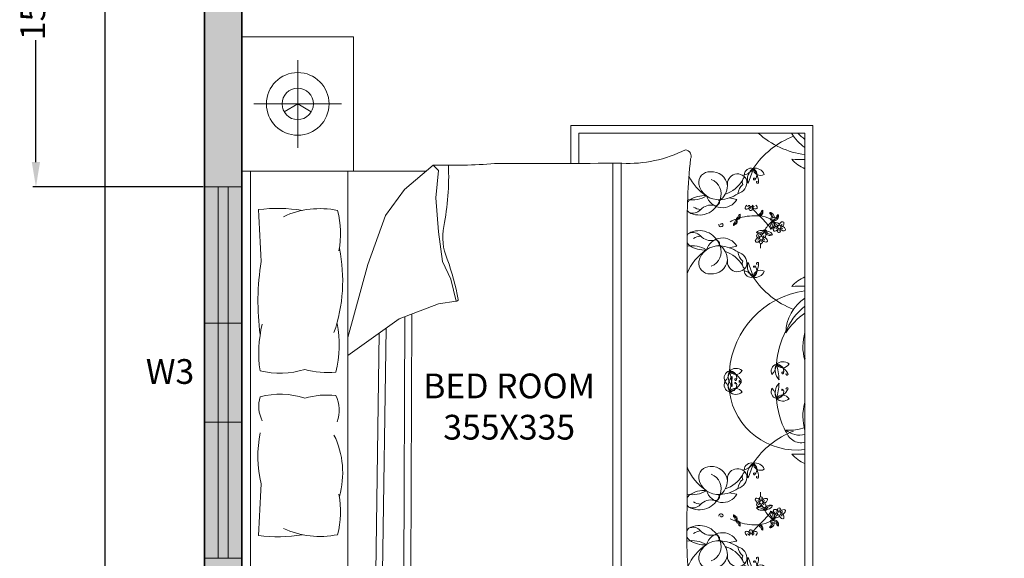
# Model space of a CAD drawing. Units: centimetres. Extents: x 2401 to 3632, y 2122 to 3526.
# Tile 2 of 10: x 2426 to 2824, y 2374 to 2591. Entities that reach past the tile are written whole.
import ezdxf

# ---------------------------------------------------------------- set-up
doc = ezdxf.new("R2010")
doc.units = ezdxf.units.CM
for name, color, linetype, lineweight in [('A-ANNO-DIMS', 9, 'Continuous', 18), ('A-ANNO-TEXT', 9, 'Continuous', 18), ('A-AREA-IDEN', 9, 'Continuous', 25), ('A-FURN', 9, 'Continuous', 18), ('A-GLAZ', 4, 'Continuous', 18), ('A-WALL', 7, 'Continuous', 35)]:
    doc.layers.add(name, color=color, linetype=linetype, lineweight=lineweight)
doc.layers.add('A-GLAZ-PATT', color=251, linetype='Continuous', lineweight=13, true_color=0x636466)
doc.layers.add('A-WALL-PATT', color=18, linetype='Continuous', lineweight=13, true_color=0x000000)
doc.styles.get("Standard").update_dxf_attribs({"font": 'arial.ttf'})
doc.dimstyles.new('ISO-25', dxfattribs={"dimtxt": 10, "dimasz": 10, "dimexe": 1.25, "dimexo": 0.625, "dimtad": 0, "dimtxsty": 'Standard', "dimcen": 2.5, "dimadec": 0, "dimazin": 0, "dimtfac": 1, "dimtmove": 0, "dimatfit": 3, "dimfxl": 1, "dimarcsym": 0})

# ---------------------------------------------------------------- blocks, each defined once
blk = doc.blocks.new('bed')
for p, q in [((3025.77, 3949.95), (3025.77, 3649.95)), ((3000.77, 3900.35), (3000.77, 3939.55)), ((2981.17, 3919.95), (3020.37, 3919.95)), ((2770.64, 3910.36), (2878.71, 3910.36)), ((2770.64, 3691.65), (2770.64, 3910.36)), ((2774.11, 3906.88), (2774.11, 3695.12)), ((2875.23, 3906.88), (2774.11, 3906.88)), ((2875.23, 3893.39), (2875.23, 3906.88)), ((2878.71, 3910.36), (2878.71, 3893.39)), ((2856.25, 3708.31), (2856.25, 3893.41)), ((2860, 3708.59), (2860, 3893.41)), ((2937.86, 3890.21), (2940.29, 3892.64)), ((2939.08, 3878.06), (2937.86, 3890.21)), ((2940.29, 3892.64), (2953.05, 3881.7)), ((3025.77, 3889.95), (2943.43, 3889.95)), ((2978.36, 3889.95), (2978.36, 3709.95)), ((3021.92, 3709.95), (3021.92, 3889.95)), ((2953.05, 3881.7), (2961.55, 3870.16)), ((2804.53, 3877.32), (2807.92, 3877.98)), ((2937.86, 3862.87), (2939.08, 3878.06)), ((2961.55, 3870.16), (2969.44, 3848.28)), ((2936.04, 3849.5), (2937.86, 3862.87)), ((2826.78, 3739.05), (2826.78, 3860.86)), ((2804.53, 3856.35), (2807.92, 3855.69)), ((2932.4, 3841.6), (2936.04, 3849.5)), ((2969.44, 3848.28), (2978.36, 3815.57)), ((2929.97, 3831.88), (2932.4, 3841.6)), ((2937.86, 3830.66), (2929.97, 3831.88)), ((2955.47, 3823.98), (2937.86, 3830.66)), ((2950.29, 3711.02), (2949.82, 3826.13)), ((2953.37, 3711.03), (2952.92, 3824.95)), ((2978.36, 3807.54), (2955.47, 3823.98)), ((2962.82, 3710.88), (2961.28, 3819.81)), ((2965.89, 3710.76), (2964.4, 3817.57)), ((2804.53, 3745.65), (2807.92, 3746.31)), ((2804.53, 3724.68), (2807.92, 3724.02)), ((2875.23, 3695.12), (2875.23, 3708.35)), ((2878.71, 3708.28), (2878.71, 3691.65)), ((3000.77, 3699.55), (3000.77, 3660.35)), ((2878.71, 3691.65), (2770.64, 3691.65)), ((2774.11, 3695.12), (2875.23, 3695.12)), ((2981.17, 3679.95), (3020.37, 3679.95))]:
    blk.add_line(p, q)
for points in [[(2975.77, 3889.95), (2975.77, 3949.95), (3025.77, 3949.95)], [(3000.77, 3919.95), (2994.7, 3916.45)], [(3000.77, 3919.95), (3006.83, 3916.45)], [(3025.77, 3709.95), (2975.77, 3709.95), (2975.77, 3649.95), (3025.77, 3649.95)], [(3000.77, 3679.95), (2994.7, 3683.45)], [(3000.77, 3679.95), (3006.83, 3683.45)]]:
    blk.add_lwpolyline(points)
for points in [[(2912.82, 3893.27, 0.001242), (2855.9, 3893.41, -0.127202), (2827.53, 3899.43)], [(3018.29, 3872.72, 0.074897), (2998.69, 3872.36, -0.472817)], [(2997.6, 3801.36, 0.14099), (3017.59, 3800.76, 0.235245)], [(2997.6, 3788.55, -0.14099), (3017.59, 3789.15, -0.235245)], [(3018.29, 3727.19, -0.074897), (2998.69, 3727.55, 0.472817)], [(2862.36, 3708.67, 0.056112), (2845.85, 3706.5, 0.095341), (2829.95, 3702.28)]]:
    blk.add_lwpolyline(points, format="xyb")
for centre, radius in [((3000.77, 3919.95), 14), ((3000.77, 3919.95), 7), ((2785.6, 3864.98), 0.764), ((2793.66, 3859.99), 0.764), ((2793.66, 3742.02), 0.764), ((2785.6, 3737.02), 0.764), ((3000.77, 3679.95), 14), ((3000.77, 3679.95), 7)]:
    blk.add_circle(centre, radius)
for centre, radius, start, end in [((2760.03, 3923.26), 23.79, 306.3036, 316.4814), ((2763.59, 3916.39), 19.09, 303.4617, 330.1116), ((2768.83, 3936.05), 39.18, 277.745, 311.8856), ((2764.96, 3869.02), 39.18, 34.3865, 68.5908), ((2827.73, 3896.66), 2.77, 93.98, 207.3412), ((2768, 3905.7), 15.93, 292.5547, 318.9546), ((2776.56, 3949.33), 54.2, 267.4081, 273.6519), ((2514.5, 3864.44), 312.3, 359.3433, 5.6887), ((2796.37, 3886.9), 4.34, 77.7115, 159.0387), ((2794.02, 3891.25), 3.27, 238.4633, 358.2869), ((2804.75, 3884.63), 9.91, 138.8402, 177.9352), ((2798.78, 3888.31), 3.2, 117.6827, 223.7762), ((2798.06, 3887.99), 3.25, 2.9516, 103.728), ((2824.04, 3897.09), 27.41, 192.5173, 207.1824), ((2793.67, 3886.12), 6.19, 345.4653, 54.2343), ((2803, 3894.63), 6.69, 211.3827, 255.2969), ((2815.84, 3882.53), 7.17, 84.9449, 172.8857), ((2816.56, 3884.61), 5.07, 354.4856, 91.0538), ((2932.84, 4167.71), 275.17, 265.8294, 271.553), ((3046.53, 3887.51), 113.22, 177.4519, 191.3392), ((2795.33, 3884.97), 0.487, 177.9352, 11.4834), ((2795.58, 3885.02), 0.236, 11.4834, 127.9409), ((2796.77, 3886.39), 0.424, 223.7762, 159.7183), ((2805.64, 3885.26), 5.62, 175.969, 254.3045), ((2804.28, 3884.18), 4.5, 350.264, 160.8688), ((2799.41, 3885.11), 2.76, 333.9755, 53.2681), ((2814.2, 3893.11), 14.16, 211.2614, 251.7045), ((2818.55, 3879.71), 6.96, 111.5819, 201.4221), ((2805.66, 3897.83), 22.71, 303.6671, 333.2997), ((2798.17, 3879.2), 5.99, 6.1662, 51.5825), ((2817.43, 3883.78), 8.71, 182.3591, 234.0401), ((2812.81, 3886.16), 9.02, 265.2933, 346.921), ((2813.05, 3893.24), 16.1, 236.2883, 266.5076), ((2810.99, 3881.04), 7.46, 209.9085, 343.1337), ((2814.13, 3876.31), 1.86, 167.3041, 285.1471), ((2819.17, 3867.4), 11.57, 122.7011, 126.3445), ((2821.34, 3879.88), 9.56, 199.2822, 299.1751), ((2824.57, 3889.51), 12.43, 238.8218, 279.1554), ((2819.17, 3867.4), 11.57, 55.785, 94.7304), ((2823.47, 3874.11), 3.61, 30.0293, 52.325), ((2789.51, 3870.54), 0.853, 56.8636, 146.9021), ((2801.41, 3872.25), 8.46, 178.3264, 187.1302), ((2792.27, 3871.07), 1.58, 11.3256, 64.4621), ((2797.62, 3873.34), 4.74, 190.2588, 210.656), ((2797.6, 3874.36), 4.82, 218.2101, 226.3071), ((2775.06, 3890.75), 28.48, 313.1541, 322.0459), ((2796.01, 3873.64), 0.586, 142.4737, 265.053), ((2796.78, 3873.76), 1.26, 127.7621, 169.0403), ((2796.11, 3874.82), 1.78, 265.053, 338.3618), ((2798.46, 3872.39), 2.32, 113.4276, 137.6104), ((2798.2, 3874.8), 0.764, 183.2768, 356.7232), ((2798.76, 3873.41), 1.25, 139.7889, 227.6792), ((2798.36, 3872.98), 0.658, 227.6792, 350.3487), ((2795.81, 3873.43), 2.5, 353.0852, 15.7171), ((2797.45, 3873.13), 1.58, 350.3487, 43.6538), ((2800.38, 3874.76), 1.84, 198.7263, 262.5032), ((2798.92, 3873.91), 0.73, 1.1081, 91.8675), ((2800.29, 3873.51), 0.59, 255.2356, 54.9248), ((2799.38, 3873.74), 1.27, 11.5637, 52.6358), ((2816.22, 3868.58), 6.15, 41.5653, 105.1471), ((2819.61, 3881.32), 8.62, 277.436, 299.9149), ((2824.18, 3875.64), 4.49, 221.5653, 293.8354), ((2823.47, 3874.11), 3.61, 314.4517, 333.558), ((3021.8, 3862.02), 40.2, 165.1039, 191.0369), ((2990.83, 3834.5), 38.67, 65.1316, 101.7583), ((5873.3, 3707.37), 2859.79, 176.68521, 177.14978), ((2785.02, 3866.54), 1.51, 157.4086, 261.4386), ((2784.17, 3866.59), 0.757, 58.0499, 135.6268), ((2783.3, 3865.19), 2.41, 14.7558, 58.0499), ((2786.72, 3869.91), 0.853, 124.3538, 214.3923), ((2787.97, 3869.78), 1.99, 190.3057, 287.1958), ((2788.54, 3870.49), 2.31, 176.9701, 248.2913), ((2805.02, 3882.67), 22.32, 212.6784, 216.3746), ((2787.76, 3869.95), 0.883, 216.3746, 291.7548), ((2795.58, 3857.56), 12.46, 124.0033, 132.4917), ((2782.77, 3855.98), 13.31, 63.7819, 68.2913), ((2789.87, 3866.22), 2.12, 128.3208, 208.8162), ((2789.87, 3869.34), 1.99, 122.8155, 187.3992), ((2788.34, 3868.51), 0.666, 289.3605, 111.7548), ((2788.84, 3868.51), 0.666, 221.8703, 44.2646), ((2791.86, 3866.57), 3.48, 157.2305, 229.0635), ((2790.75, 3869.08), 2.31, 109.4799, 177.6828), ((2790.69, 3867.72), 2.05, 174.4544, 220.6188), ((2779.03, 3856.28), 14.94, 30.544, 49.818), ((2789.95, 3869.59), 0.883, 148.8844, 224.2646), ((2808.3, 3858.51), 22.32, 145.1882, 148.8844), ((2795.58, 3857.56), 12.46, 94.756, 119.2041), ((2822.1, 3839.62), 40.99, 132.2412, 142.1744), ((2794.44, 3871.41), 1.44, 188.3432, 274.2869), ((2795.7, 3872.2), 2.51, 210.656, 242.6341), ((2794.04, 3870.31), 0.611, 325.7657, 67.4417), ((2796.2, 3845.18), 24.85, 73.5842, 93.8277), ((2811.5, 3870.46), 8.46, 178.3264, 187.1302), ((2802.37, 3869.29), 1.58, 11.3256, 64.4621), ((2807.71, 3871.55), 4.74, 190.2588, 210.656), ((2804.53, 3869.62), 1.44, 188.3432, 274.2869), ((2805.8, 3870.42), 2.51, 210.656, 242.6341), ((2807.7, 3872.58), 4.82, 218.2101, 226.3071), ((2804.13, 3868.53), 0.611, 325.7657, 67.4417), ((2805.85, 3867.41), 1.44, 147.5332, 233.4768), ((2804.7, 3867.58), 0.611, 354.3784, 96.0543), ((2807.15, 3868.15), 2.51, 179.1859, 211.164), ((2796.2, 3845.18), 24.85, 63.0032, 69.8941), ((2809.96, 3868.8), 4.82, 195.5129, 203.6099), ((2783.42, 3863.83), 0.586, 142.4737, 265.053), ((2784.19, 3863.94), 1.26, 61.2196, 169.0403), ((2783.52, 3865.01), 1.78, 265.053, 338.3618), ((2785.87, 3862.58), 2.32, 113.4276, 137.6104), ((2784.96, 3866.11), 0.506, 172.906, 277.132), ((2786.17, 3863.6), 1.25, 139.7889, 227.6792), ((2785.77, 3863.16), 0.658, 227.6792, 350.3487), ((2786.67, 3865.83), 1.04, 36.1046, 181.4281), ((2783.22, 3863.62), 2.5, 353.0852, 15.7171), ((2784.86, 3863.32), 1.58, 350.3487, 43.6538), ((2787.79, 3864.95), 1.84, 198.7263, 262.5032), ((2786.06, 3866.65), 1.05, 270.0645, 331.1507), ((2786.96, 3866.4), 1.2, 221.8413, 265.7877), ((2786.33, 3864.09), 0.73, 1.1081, 91.8675), ((2786.95, 3865.94), 0.749, 263.7526, 41.7054), ((2786.79, 3863.93), 1.27, 11.5637, 86.365), ((2787.7, 3863.7), 0.59, 255.2356, 54.9248), ((2790.26, 3866.38), 2.53, 207.7043, 254.3516), ((2788.61, 3864.93), 3.48, 270.278, 342.111), ((2790.93, 3860.58), 2.46, 98.7227, 159.3375), ((2787.26, 3864.79), 2.46, 340.0041, 40.6188), ((2790.25, 3865.04), 2.05, 278.7227, 324.8872), ((2789.89, 3863.37), 2.12, 290.5253, 358.5375), ((2794.02, 3863.97), 2.12, 182.8499, 266.1226), ((2793.19, 3865.47), 2.05, 231.7607, 277.9252), ((2794.79, 3865.83), 3.48, 214.5369, 286.3699), ((2793.81, 3861), 2.46, 37.3105, 97.9252), ((2809.06, 3869.3), 4.74, 211.164, 231.5612), ((2809.89, 3873.16), 8.46, 234.6898, 243.4936), ((2804.54, 3865.66), 1.58, 357.3579, 50.4944), ((2811.3, 3865.97), 0.578, 12.7051, 190.4384), ((2811.66, 3866.04), 0.94, 190.4384, 10.4136), ((2821.34, 3853.79), 9.56, 60.8249, 160.7178), ((2911.57, 3860.44), 24.42, 336.2616, 11.3392), ((2789.7, 3863.74), 2.53, 244.9899, 291.6373), ((2791.47, 3858.83), 0.586, 142.4737, 265.053), ((2792.24, 3858.95), 1.26, 61.2196, 169.0403), ((2791.57, 3860.01), 1.78, 265.053, 338.3618), ((2793.07, 3861.54), 1.51, 157.4086, 261.4386), ((2792.22, 3861.59), 0.757, 58.0499, 135.6268), ((2793.92, 3857.58), 2.32, 113.4276, 137.6104), ((2793.01, 3861.12), 0.506, 172.906, 277.132), ((2791.35, 3860.19), 2.41, 14.7558, 58.0499), ((2779.03, 3856.28), 14.94, 23.0501, 23.8477), ((2794.22, 3858.6), 1.25, 139.7889, 227.6792), ((2794.72, 3860.83), 1.04, 36.1046, 181.4281), ((2791.27, 3858.62), 2.5, 353.0852, 15.7171), ((2794.09, 3864.38), 2.53, 265.0106, 311.658), ((2792.91, 3858.32), 1.58, 350.3487, 43.6538), ((2795.84, 3859.95), 1.84, 198.7263, 262.5032), ((2794.11, 3861.65), 1.05, 270.0645, 331.1507), ((2795.01, 3861.4), 1.2, 221.8413, 265.7877), ((2794.38, 3859.1), 0.73, 1.1081, 91.8675), ((2795, 3860.95), 0.749, 263.7526, 41.7054), ((2794.84, 3858.93), 1.27, 11.5637, 86.365), ((2795.75, 3858.7), 0.59, 255.2356, 54.9248), ((2810.99, 3852.63), 7.46, 16.8663, 150.0915), ((2814.13, 3857.35), 1.86, 74.8529, 192.6959), ((2816.22, 3865.09), 6.15, 254.8529, 318.4347), ((2819.61, 3852.35), 8.62, 60.0851, 82.564), ((2824.18, 3858.03), 4.49, 66.1646, 138.4347), ((2823.47, 3859.56), 3.61, 23.229, 45.5483), ((2793.82, 3858.17), 0.658, 227.6792, 350.3487), ((2779.03, 3856.28), 14.94, 357.1071, 4.7585), ((2805.64, 3848.41), 5.62, 105.6955, 184.031), ((2798.17, 3854.46), 5.99, 308.4175, 353.8338), ((2814.2, 3840.56), 14.16, 108.2955, 148.7386), ((2813.05, 3840.43), 16.1, 93.4924, 123.7117), ((2817.43, 3849.89), 8.71, 125.9599, 177.6409), ((2818.55, 3853.96), 6.96, 158.5779, 248.4181), ((2812.81, 3847.51), 9.02, 13.079, 94.7067), ((2819.17, 3866.26), 11.57, 233.6555, 237.2989), ((2824.57, 3844.16), 12.43, 79.7133, 121.1782), ((2819.17, 3866.26), 11.57, 265.2696, 304.215), ((2805.66, 3835.83), 22.71, 21.4941, 56.3329), ((2823.47, 3859.56), 3.61, 307.675, 336.7144), ((3050.38, 3840.86), 69.73, 168.0397, 199.2615), ((2804.28, 3849.49), 4.5, 199.1312, 9.736), ((2799.41, 3848.56), 2.76, 306.7319, 26.0245), ((2815.84, 3851.14), 7.17, 187.1143, 275.0551), ((2816.56, 3849.06), 5.07, 268.9462, 5.5144), ((3043.34, 3811.05), 116.34, 160.1194, 169.3383), ((2909.73, 3831.62), 108.8, 352.2196, 9.497), ((2794.02, 3842.42), 3.27, 1.7131, 121.5367), ((2796.37, 3846.77), 4.34, 200.9613, 282.2885), ((2795.33, 3848.7), 0.487, 348.5166, 182.0648), ((2804.75, 3849.04), 9.91, 182.0648, 221.1598), ((2795.58, 3848.65), 0.236, 232.0591, 348.5166), ((2798.78, 3845.36), 3.2, 136.2238, 242.3173), ((2796.93, 3847.24), 0.255, 200.2667, 136.2271), ((2793.67, 3847.55), 6.19, 305.7657, 14.5347), ((2824.04, 3836.58), 27.41, 152.8176, 167.4827), ((2798.06, 3845.68), 3.25, 256.272, 357.0484), ((2803, 3839.04), 6.69, 104.7031, 148.6173), ((2768, 3827.97), 15.93, 41.0454, 67.4453), ((2764.96, 3864.65), 39.18, 291.4092, 325.6135), ((2776.56, 3784.33), 54.2, 86.3481, 92.5919), ((2768.83, 3797.62), 39.18, 4.4623, 82.255), ((2763.59, 3817.28), 19.09, 1.272, 56.5383), ((2929.73, 3832.56), 0.724, 178.8623, 289.7536), ((2760.03, 3810.41), 23.79, 17.8504, 53.6964), ((2753.34, 3797.91), 35.39, 34.0123, 54.053), ((2747.85, 3800.62), 39.18, 4.4623, 27.4146), ((3035.15, 3812.63), 52.9, 169.8617, 193.6238), ((2964.72, 3808.64), 53.46, 351.5249, 13.96), ((2753.52, 3811.58), 21.54, 343.5431, 17.0202), ((2742.41, 3803.04), 31.85, 4.3787, 5.6357), ((2720.59, 3786.27), 56.92, 19.7217, 19.9028), ((2783.99, 3800.45), 4.34, 47.7873, 129.1145), ((2784.12, 3805.39), 3.27, 208.5391, 328.3627), ((2790.12, 3794.3), 9.91, 108.9159, 148.011), ((2786.78, 3800.47), 3.2, 87.7585, 193.852), ((2813.06, 3795.47), 27.41, 162.593, 177.2582), ((2781.26, 3801.12), 6.19, 315.5411, 24.3101), ((2793.6, 3803.84), 6.69, 181.4585, 225.3727), ((2786, 3800.55), 3.25, 333.0274, 73.8037), ((2804.97, 3797.45), 4.34, 47.7873, 129.1145), ((2987.57, 3836.72), 36.76, 264.0129, 285.8293), ((2782.13, 3799.29), 0.487, 148.011, 341.5592), ((2782.37, 3799.21), 0.236, 341.5592, 98.0167), ((2784.08, 3799.8), 0.424, 193.852, 129.9245), ((2805.11, 3802.39), 3.27, 208.5391, 328.3627), ((2811.1, 3791.3), 9.91, 108.9159, 148.011), ((2807.77, 3797.47), 3.2, 87.7585, 193.852), ((2805.07, 3796.8), 0.424, 193.852, 129.9245), ((2802.25, 3798.12), 6.19, 315.5411, 24.3101), ((2834.04, 3792.47), 27.41, 162.593, 177.2582), ((2802.25, 3793.88), 6.19, 335.6899, 44.4589), ((2834.04, 3799.53), 27.41, 182.7418, 197.407), ((2806.98, 3797.55), 3.25, 333.0274, 73.8037), ((2814.58, 3800.84), 6.69, 181.4585, 225.3727), ((2782.13, 3792.71), 0.487, 18.4408, 211.989), ((2790.12, 3797.71), 9.91, 211.989, 251.0841), ((2782.37, 3792.79), 0.236, 261.9833, 18.4408), ((2786.78, 3791.54), 3.2, 166.148, 272.2415), ((2784.25, 3792.24), 0.255, 230.1909, 166.0209), ((2813.06, 3796.53), 27.41, 182.7418, 197.407), ((2781.26, 3790.88), 6.19, 335.6899, 44.4589), ((2793.6, 3788.16), 6.69, 134.6273, 178.5415), ((2786, 3791.45), 3.25, 286.1963, 26.9726), ((2805.11, 3789.62), 3.27, 31.6373, 151.4609), ((2803.11, 3796.29), 0.487, 148.011, 341.5592), ((2803.11, 3795.71), 0.487, 18.4408, 211.989), ((2811.1, 3800.7), 9.91, 211.989, 251.0841), ((2803.35, 3796.21), 0.236, 341.5592, 98.0167), ((2803.35, 3795.79), 0.236, 261.9833, 18.4408), ((2807.77, 3794.53), 3.2, 166.148, 272.2415), ((2805.23, 3795.24), 0.255, 230.1909, 166.0209), ((2806.98, 3794.45), 3.25, 286.1963, 26.9726), ((2814.58, 3791.16), 6.69, 134.6273, 178.5415), ((2777.88, 3795.65), 30.32, 262.8636, 351.8197), ((2784.12, 3786.62), 3.27, 31.6373, 151.4609), ((2783.99, 3791.55), 4.34, 230.8855, 312.2127), ((2747.85, 3791.38), 39.18, 332.5854, 355.5377), ((2804.97, 3794.55), 4.34, 230.8855, 312.2127), ((2998.15, 3783.03), 15.9, 155.0183, 198.5407), ((2987.57, 3753.18), 36.76, 74.1707, 95.9871), ((3003.33, 3785.03), 14.84, 333.3437, 16.1026), ((2753.52, 3780.42), 21.54, 342.9798, 16.4569), ((2742.41, 3788.96), 31.85, 354.3643, 355.6213), ((2720.59, 3805.74), 56.92, 340.0972, 340.2783), ((2780.65, 3791.73), 17.54, 248.117, 276.6195), ((2775.77, 3775.64), 7.03, 256.3898, 349.0739), ((2776.73, 3780.92), 8.89, 252.8609, 311.9049), ((2764.96, 3737.36), 39.18, 34.3865, 68.5908), ((3018.84, 3755.24), 38.19, 153.8761, 196.1746), ((2965.8, 3762.79), 52.74, 346.3427, 11.1841), ((2776.56, 3817.67), 54.2, 267.4081, 273.6519), ((2768, 3774.04), 15.93, 292.5547, 318.9546), ((2796.37, 3755.24), 4.34, 77.7115, 159.0387), ((2794.02, 3759.58), 3.27, 238.4633, 358.2869), ((2804.75, 3752.96), 9.91, 138.8402, 177.9352), ((2798.78, 3756.64), 3.2, 117.6827, 223.7762), ((2798.06, 3756.33), 3.25, 2.9516, 103.728), ((2803, 3762.97), 6.69, 211.3827, 255.2969), ((2793.67, 3754.46), 6.19, 345.4653, 54.2343), ((2824.04, 3765.42), 27.41, 192.5173, 207.1824), ((2804.28, 3752.51), 4.5, 350.264, 160.8688), ((2815.84, 3750.86), 7.17, 84.9449, 172.8857), ((2816.56, 3752.94), 5.07, 354.4856, 91.0538), ((2805.66, 3766.17), 22.71, 303.6671, 338.5059), ((2795.33, 3753.3), 0.487, 177.9352, 11.4834), ((2795.58, 3753.35), 0.236, 11.4834, 127.9409), ((2796.77, 3754.72), 0.424, 223.7762, 159.7183), ((2805.64, 3753.59), 5.62, 175.969, 254.3045), ((2799.41, 3753.44), 2.76, 333.9755, 53.2681), ((2814.2, 3761.44), 14.16, 211.2614, 251.7045), ((2818.55, 3748.05), 6.96, 111.5819, 201.4221), ((2798.17, 3747.54), 5.99, 6.1662, 51.5825), ((2813.05, 3761.57), 16.1, 236.2883, 266.5076), ((2817.43, 3752.11), 8.71, 182.3591, 234.0401), ((2812.81, 3754.5), 9.02, 265.2933, 346.921), ((5873.3, 3892.54), 2859.79, 182.85022, 183.31479), ((2794.22, 3743.4), 1.25, 132.3208, 220.2111), ((2793.82, 3743.84), 0.658, 9.6513, 132.3208), ((2779.03, 3745.73), 14.94, 355.2415, 2.8929), ((2792.91, 3743.68), 1.58, 316.3462, 9.6513), ((2795.84, 3742.05), 1.84, 97.4968, 161.2737), ((2795.75, 3743.3), 0.59, 305.0752, 104.7644), ((2810.99, 3749.37), 7.46, 209.9085, 343.1337), ((2814.13, 3744.65), 1.86, 167.3041, 285.1471), ((2819.17, 3735.74), 11.57, 122.7011, 126.3445), ((2821.34, 3748.21), 9.56, 199.2822, 299.1751), ((2824.57, 3757.84), 12.43, 238.8218, 280.2867), ((2819.17, 3735.74), 11.57, 55.785, 94.7304), ((2823.47, 3742.45), 3.61, 23.2856, 52.325), ((3021.8, 3737.89), 40.2, 168.9631, 194.8961), ((2785.77, 3738.84), 0.658, 9.6513, 132.3208), ((2789.7, 3738.26), 2.53, 68.3627, 115.0101), ((2788.61, 3737.07), 3.48, 17.889, 89.722), ((2790.93, 3741.42), 2.46, 200.6625, 261.2773), ((2789.89, 3738.63), 2.12, 1.4625, 69.4747), ((2791.47, 3743.17), 0.586, 94.947, 217.5263), ((2792.24, 3743.06), 1.26, 190.9597, 298.7804), ((2791.57, 3741.99), 1.78, 21.6382, 94.947), ((2793.07, 3740.46), 1.51, 98.5614, 202.5914), ((2792.22, 3740.41), 0.757, 224.3732, 301.9501), ((2794.02, 3738.03), 2.12, 93.8774, 177.1501), ((2794.79, 3736.17), 3.48, 73.6301, 145.4631), ((2793.92, 3744.42), 2.32, 222.3896, 246.5724), ((2793.01, 3740.89), 0.506, 82.868, 187.094), ((2791.35, 3741.81), 2.41, 301.9501, 345.2442), ((2779.03, 3745.73), 14.94, 336.1523, 336.9499), ((2793.81, 3741), 2.46, 262.0748, 322.6895), ((2791.27, 3743.38), 2.5, 344.2829, 6.9148), ((2794.72, 3741.17), 1.04, 178.5719, 323.8954), ((2794.09, 3737.62), 2.53, 48.342, 94.9894), ((2795.01, 3740.6), 1.2, 94.2123, 138.1587), ((2794.11, 3740.35), 1.05, 28.8493, 89.9355), ((2794.38, 3742.91), 0.73, 268.1325, 358.8919), ((2794.84, 3743.07), 1.27, 273.635, 348.4363), ((2795, 3741.06), 0.749, 318.2946, 96.2474), ((2816.22, 3736.91), 6.15, 41.5653, 105.1471), ((2819.61, 3749.66), 8.62, 277.436, 299.9149), ((2824.18, 3743.97), 4.49, 221.5653, 293.8354), ((2823.47, 3742.45), 3.61, 314.4517, 336.7144), ((2783.42, 3738.18), 0.586, 94.947, 217.5263), ((2784.19, 3738.06), 1.26, 190.9597, 298.7804), ((2783.52, 3736.99), 1.78, 21.6382, 94.947), ((2785.02, 3735.46), 1.51, 98.5614, 202.5914), ((2785.87, 3739.42), 2.32, 222.3896, 246.5724), ((2784.96, 3735.89), 0.506, 82.868, 187.094), ((2783.3, 3736.82), 2.41, 301.9501, 345.2442), ((2786.17, 3738.4), 1.25, 132.3208, 220.2111), ((2783.22, 3738.38), 2.5, 344.2829, 6.9148), ((2786.67, 3736.18), 1.04, 178.5719, 323.8954), ((2784.86, 3738.68), 1.58, 316.3462, 9.6513), ((2787.79, 3737.05), 1.84, 97.4968, 161.2737), ((2786.96, 3735.61), 1.2, 94.2123, 138.1587), ((2786.06, 3735.36), 1.05, 28.8493, 89.9355), ((2786.33, 3737.91), 0.73, 268.1325, 358.8919), ((2786.79, 3738.08), 1.27, 273.635, 348.4363), ((2786.95, 3736.06), 0.749, 318.2946, 96.2474), ((2795.58, 3744.44), 12.46, 227.5083, 235.9967), ((2787.7, 3738.3), 0.59, 305.0752, 104.7644), ((2789.87, 3735.78), 2.12, 151.1838, 231.6792), ((2790.26, 3735.62), 2.53, 105.6484, 152.2957), ((2791.86, 3735.43), 3.48, 130.9365, 202.7695), ((2790.69, 3734.28), 2.05, 139.3812, 185.5456), ((2779.03, 3745.73), 14.94, 310.182, 329.456), ((2787.26, 3737.22), 2.46, 319.3812, 19.9959), ((2822.1, 3762.38), 40.99, 217.8256, 227.7588), ((2790.25, 3736.96), 2.05, 35.1128, 81.2773), ((2793.19, 3736.53), 2.05, 82.0748, 128.2393), ((2805.85, 3734.59), 1.44, 126.5232, 212.4668), ((2807.15, 3733.85), 2.51, 148.836, 180.8141), ((2809.06, 3732.7), 4.74, 128.4388, 148.836), ((2809.89, 3728.84), 8.46, 116.5064, 125.3102), ((2809.96, 3733.2), 4.82, 156.3901, 164.4871), ((2804.54, 3736.34), 1.58, 309.5056, 2.6421), ((2811.3, 3736.03), 0.578, 169.5616, 347.2949), ((2811.66, 3735.96), 0.94, 349.5864, 169.5616), ((2535.01, 3729.86), 291.92, 355.2402, 1.8035), ((2784.17, 3735.41), 0.757, 224.3732, 301.9501), ((2786.72, 3732.09), 0.853, 145.6077, 235.6462), ((2787.97, 3732.22), 1.99, 72.8042, 169.6943), ((2788.54, 3731.51), 2.31, 111.7087, 183.0299), ((2805.02, 3719.34), 22.32, 143.6254, 147.3216), ((2787.76, 3732.05), 0.883, 68.2452, 143.6254), ((2782.77, 3746.02), 13.31, 291.7087, 296.2181), ((2789.87, 3732.67), 1.99, 172.6008, 237.1845), ((2788.34, 3733.49), 0.666, 248.2452, 70.6395), ((2788.84, 3733.49), 0.666, 315.7354, 138.1297), ((2790.75, 3732.92), 2.31, 182.3172, 250.5201), ((2789.51, 3731.46), 0.853, 213.0979, 303.1364), ((2789.95, 3732.41), 0.883, 135.7354, 211.1156), ((2808.3, 3743.49), 22.32, 211.1156, 214.8118), ((2795.58, 3744.44), 12.46, 240.7959, 265.244), ((2797.62, 3728.66), 4.74, 149.344, 169.7412), ((2801.41, 3729.75), 8.46, 172.8698, 181.6736), ((2792.27, 3730.93), 1.58, 295.5379, 348.6744), ((2794.44, 3730.6), 1.44, 85.7131, 171.6568), ((2795.7, 3729.8), 2.51, 117.3659, 149.344), ((2797.6, 3727.64), 4.82, 133.6929, 141.7899), ((2794.04, 3731.69), 0.611, 292.5583, 34.2343), ((2796.2, 3756.82), 24.85, 266.1723, 286.4158), ((2775.06, 3711.25), 28.48, 37.9541, 46.8459), ((2811.5, 3731.54), 8.46, 172.8698, 181.6736), ((2807.71, 3730.45), 4.74, 149.344, 169.7412), ((2802.37, 3732.72), 1.58, 295.5379, 348.6744), ((2804.53, 3732.38), 1.44, 85.7131, 171.6568), ((2805.8, 3731.59), 2.51, 117.3659, 149.344), ((2807.7, 3729.43), 4.82, 133.6929, 141.7899), ((2804.13, 3733.47), 0.611, 292.5583, 34.2343), ((2804.7, 3734.43), 0.611, 263.9457, 5.6216), ((2796.2, 3756.82), 24.85, 290.1059, 296.9968), ((2821.34, 3722.12), 9.56, 60.8249, 160.7178), ((2824.18, 3726.36), 4.49, 66.1646, 138.4347), ((2796.01, 3728.36), 0.586, 94.947, 217.5263), ((2796.78, 3728.25), 1.26, 190.9597, 232.2379), ((2796.11, 3727.18), 1.78, 21.6382, 94.947), ((2798.46, 3729.61), 2.32, 222.3896, 246.5724), ((2798.2, 3727.21), 0.764, 3.2768, 176.7232), ((2798.76, 3728.59), 1.25, 132.3208, 220.2111), ((2798.36, 3729.03), 0.658, 9.6513, 132.3208), ((2795.81, 3728.57), 2.5, 344.2829, 6.9148), ((2797.45, 3728.87), 1.58, 316.3462, 9.6513), ((2800.38, 3727.24), 1.84, 97.4968, 161.2737), ((2798.92, 3728.1), 0.73, 268.1325, 358.8919), ((2800.29, 3728.49), 0.59, 305.0752, 104.7644), ((2799.38, 3728.26), 1.27, 307.3642, 348.4363), ((2810.99, 3720.97), 7.46, 16.8663, 150.0915), ((2814.13, 3725.69), 1.86, 74.8529, 192.6959), ((2816.22, 3733.42), 6.15, 254.8529, 318.4347), ((2819.61, 3720.68), 8.62, 60.0851, 82.564), ((2823.47, 3727.89), 3.61, 307.675, 342.5814), ((2823.47, 3727.89), 3.61, 16.6343, 45.5483), ((2990.83, 3765.41), 38.67, 258.2417, 294.8684), ((2805.64, 3716.74), 5.62, 105.6955, 184.031), ((2798.17, 3722.8), 5.99, 308.4175, 353.8338), ((2814.2, 3708.9), 14.16, 108.2955, 148.7386), ((2813.05, 3708.76), 16.1, 93.4924, 123.7117), ((2817.43, 3718.23), 8.71, 125.9599, 177.6409), ((2818.55, 3722.29), 6.96, 158.5779, 248.4181), ((2812.81, 3715.84), 9.02, 13.079, 94.7067), ((2819.17, 3734.6), 11.57, 233.6555, 237.2989), ((2824.57, 3712.5), 12.43, 79.249, 121.1782), ((2819.17, 3734.6), 11.57, 265.2696, 304.215), ((2805.66, 3704.17), 22.71, 23.6453, 56.3329), ((2795.33, 3717.04), 0.487, 348.5166, 182.0648), ((2824.04, 3704.91), 27.41, 152.8176, 167.4827), ((2793.67, 3715.88), 6.19, 305.7657, 14.5347), ((2804.28, 3717.82), 4.5, 199.1312, 9.736), ((2799.41, 3716.9), 2.76, 306.7319, 26.0245), ((2815.84, 3719.47), 7.17, 187.1143, 275.0551), ((2816.56, 3717.4), 5.07, 268.9462, 5.5144), ((2794.02, 3710.76), 3.27, 1.7131, 121.5367), ((2796.37, 3715.1), 4.34, 200.9613, 282.2885), ((2804.75, 3717.37), 9.91, 182.0648, 221.1598), ((2795.58, 3716.99), 0.236, 232.0591, 348.5166), ((2798.78, 3713.69), 3.2, 136.2238, 242.3173), ((2796.93, 3715.57), 0.255, 200.2667, 136.2271), ((2803, 3707.37), 6.69, 104.7031, 148.6173), ((2798.06, 3714.01), 3.25, 256.272, 357.0484), ((2768, 3696.3), 15.93, 41.0454, 67.4453), ((2764.96, 3732.98), 39.18, 291.4092, 325.6135), ((2922.1, 3008.05), 703.17, 89.11454, 94.87351), ((2941.69, 3172.15), 539.05, 86.1, 90.9282), ((2776.56, 3652.67), 54.2, 86.3481, 92.5919), ((2768.83, 3665.96), 39.18, 48.1144, 82.255), ((2828.43, 3704.55), 2.73, 156.5219, 303.8264), ((2763.59, 3685.61), 19.09, 29.8884, 56.5383), ((2760.03, 3678.74), 23.79, 43.5186, 53.6964)]:
    blk.add_arc(centre, radius, start, end)
blk = doc.blocks.new('*D12')
at = {"layer": 'A-ANNO-DIMS', "color": 0, "lineweight": -2, "transparency": 16777216}
for p, q in [((2499.81, 3451.1), (2458.94, 3451.1)), ((2460.19, 3441.1), (2460.19, 2873.73)), ((2460.19, 2276.1), (2460.19, 2843.48)), ((2499.81, 2266.1), (2458.94, 2266.1))]:
    blk.add_line(p, q, dxfattribs=at)
at = {"layer": 'A-ANNO-DIMS', "color": 0, "transparency": 16777216}
for points in [[(2458.52, 3441.1), (2461.85, 3441.1), (2460.19, 3451.1)], [(2458.52, 2276.1), (2461.85, 2276.1), (2460.19, 2266.1)]]:
    blk.add_solid(points, dxfattribs=at)
at = {"layer": 'Defpoints', "color": 0, "transparency": 16777216}
for p in [(2500.44, 3451.1), (2460.19, 2266.1), (2500.44, 2266.1)]:
    blk.add_point(p, dxfattribs=at)
at = {"layer": 'A-ANNO-DIMS', "color": 0, "transparency": 16777216, "insert": (2460.19, 2858.6), "char_height": 10, "attachment_point": 5, "rotation": 90}
blk.add_mtext('1185', dxfattribs=at)
blk = doc.blocks.new('WIN-1500-3P')
for p, q in [((0, 15), (0, 0)), ((55, 15), (55, 0)), ((95, 15), (95, 0)), ((150, 15), (150, 0)), ((0, 9.5), (150, 9.5)), ((0, 5.5), (150, 5.5))]:
    blk.add_line(p, q)
blk = doc.blocks.new('*D40')
at = {"layer": 'A-ANNO-DIMS', "color": 0, "lineweight": -2, "transparency": 16777216}
for p, q in [((2499.81, 2676.1), (2431.04, 2676.1)), ((2432.29, 2666.1), (2432.29, 2616.92)), ((2432.29, 2533.6), (2432.29, 2582.79)), ((2499.81, 2523.6), (2431.04, 2523.6))]:
    blk.add_line(p, q, dxfattribs=at)
at = {"layer": 'A-ANNO-DIMS', "color": 0, "transparency": 16777216}
for points in [[(2430.62, 2666.1), (2433.95, 2666.1), (2432.29, 2676.1)], [(2430.62, 2533.6), (2433.95, 2533.6), (2432.29, 2523.6)]]:
    blk.add_solid(points, dxfattribs=at)
at = {"layer": 'Defpoints', "color": 0, "transparency": 16777216}
for p in [(2432.29, 2676.1), (2500.44, 2676.1), (2500.44, 2523.6)]:
    blk.add_point(p, dxfattribs=at)
at = {"layer": 'A-ANNO-DIMS', "color": 0, "transparency": 16777216, "insert": (2432.29, 2599.85), "char_height": 10, "attachment_point": 5, "rotation": 90}
blk.add_mtext('152.5', dxfattribs=at)

msp = doc.modelspace()

# ---------------------------------------------------------------- hatches: boundary and pattern name
at = {"layer": 'A-GLAZ-PATT'}
h = msp.add_hatch(color=256, dxfattribs=at)
h.dxf.hatch_style = 1
h.paths.add_polyline_path([(2505.936, 3356.104), (2500.436, 3356.104), (2500.436, 3301.104), (2505.936, 3301.104)])
h.paths.add_polyline_path([(2509.936, 3356.104), (2505.936, 3356.104), (2505.936, 3301.104), (2509.936, 3301.104)])
h.paths.add_polyline_path([(2515.436, 3335.674), (2515.436, 3356.104), (2509.936, 3356.104), (2509.936, 3301.104), (2515.436, 3301.104)])
h.paths.add_polyline_path([(2509.936, 3301.104), (2505.936, 3301.104), (2505.936, 3261.104), (2509.936, 3261.104)])
h.paths.add_polyline_path([(2515.436, 3301.104), (2509.936, 3301.104), (2509.936, 3261.104), (2515.436, 3261.104)])
h.paths.add_polyline_path([(2505.936, 3301.104), (2500.436, 3301.104), (2500.436, 3261.104), (2505.936, 3261.104)])
h.paths.add_polyline_path([(2515.436, 3261.104), (2509.936, 3261.104), (2509.936, 3206.104), (2515.436, 3206.104)])
h.paths.add_polyline_path([(2505.936, 3261.104), (2500.436, 3261.104), (2500.436, 3206.104), (2505.936, 3206.104)])
h.paths.add_polyline_path([(2509.936, 3261.104), (2505.936, 3261.104), (2505.936, 3206.104), (2509.936, 3206.104)])
h.paths.add_polyline_path([(3127.936, 3451.104), (3072.936, 3451.104), (3072.936, 3445.604), (3127.936, 3445.604)])
h.paths.add_polyline_path([(3032.936, 3441.604), (2977.936, 3441.604), (2977.936, 3436.104), (3032.936, 3436.104)])
h.paths.add_polyline_path([(3032.936, 3451.104), (2977.936, 3451.104), (2977.936, 3445.604), (3032.936, 3445.604)])
h.paths.add_polyline_path([(3032.936, 3445.604), (2977.936, 3445.604), (2977.936, 3441.604), (3032.936, 3441.604)])
h.paths.add_polyline_path([(3072.936, 3451.104), (3032.936, 3451.104), (3032.936, 3445.604), (3072.936, 3445.604)])
h.paths.add_polyline_path([(3072.936, 3445.604), (3032.936, 3445.604), (3032.936, 3441.604), (3072.936, 3441.604)])
h.paths.add_polyline_path([(3072.936, 3441.604), (3032.936, 3441.604), (3032.936, 3436.104), (3072.936, 3436.104)])
h.paths.add_polyline_path([(3127.936, 3441.604), (3072.936, 3441.604), (3072.936, 3436.104), (3127.936, 3436.104)])
h.paths.add_polyline_path([(3127.936, 3445.604), (3072.936, 3445.604), (3072.936, 3441.604), (3127.936, 3441.604)])
h.paths.add_polyline_path([(3245.436, 3356.104), (3239.936, 3356.104), (3239.936, 3301.104), (3245.436, 3301.104)])
h.paths.add_polyline_path([(3239.936, 3356.104), (3235.936, 3356.104), (3235.936, 3301.104), (3239.936, 3301.104)])
h.paths.add_polyline_path([(3235.936, 3356.104), (3230.436, 3356.104), (3230.436, 3301.104), (3235.936, 3301.104)])
h.paths.add_polyline_path([(3235.936, 3301.104), (3230.436, 3301.104), (3230.436, 3261.104), (3235.936, 3261.104)])
h.paths.add_polyline_path([(3239.936, 3301.104), (3235.936, 3301.104), (3235.936, 3261.104), (3239.936, 3261.104)])
h.paths.add_polyline_path([(3245.436, 3301.104), (3239.936, 3301.104), (3239.936, 3261.104), (3245.436, 3261.104)])
h.paths.add_polyline_path([(3245.436, 3261.104), (3239.936, 3261.104), (3239.936, 3206.104), (3245.436, 3206.104)])
h.paths.add_polyline_path([(3239.936, 3261.104), (3235.936, 3261.104), (3235.936, 3206.104), (3239.936, 3206.104)])
h.paths.add_polyline_path([(3235.936, 3261.104), (3230.436, 3261.104), (3230.436, 3206.104), (3235.936, 3206.104)])
h.paths.add_polyline_path([(3239.936, 3036.104), (3235.936, 3036.104), (3235.936, 2976.104), (3239.936, 2976.104)])
h.paths.add_polyline_path([(3235.936, 3036.104), (3230.436, 3036.104), (3230.436, 2976.104), (3235.936, 2976.104)])
h.paths.add_polyline_path([(3245.436, 3036.104), (3239.936, 3036.104), (3239.936, 2976.104), (3245.436, 2976.104)])
h.paths.add_polyline_path([(3235.936, 2836.104), (3230.436, 2836.104), (3230.436, 2781.104), (3235.936, 2781.104)])
h.paths.add_polyline_path([(3245.436, 2836.104), (3239.936, 2836.104), (3239.936, 2781.104), (3245.436, 2781.104)])
h.paths.add_polyline_path([(3239.936, 2836.104), (3235.936, 2836.104), (3235.936, 2781.104), (3239.936, 2781.104)])
h.paths.add_polyline_path([(3245.436, 2781.104), (3239.936, 2781.104), (3239.936, 2741.104), (3245.436, 2741.104)])
h.paths.add_polyline_path([(3239.936, 2781.104), (3235.936, 2781.104), (3235.936, 2741.104), (3239.936, 2741.104)])
h.paths.add_polyline_path([(3235.936, 2781.104), (3230.436, 2781.104), (3230.436, 2741.104), (3235.936, 2741.104)])
h.paths.add_polyline_path([(3245.436, 2741.104), (3239.936, 2741.104), (3239.936, 2686.104), (3245.436, 2686.104)])
h.paths.add_polyline_path([(3239.936, 2741.104), (3235.936, 2741.104), (3235.936, 2686.104), (3239.936, 2686.104)])
h.paths.add_polyline_path([(3235.936, 2741.104), (3230.436, 2741.104), (3230.436, 2686.104), (3235.936, 2686.104)])
h.paths.add_polyline_path([(3187.936, 2606.104), (3132.936, 2606.104), (3132.936, 2600.604), (3187.936, 2600.604)])
h.paths.add_polyline_path([(3187.936, 2600.604), (3132.936, 2600.604), (3132.936, 2596.604), (3187.936, 2596.604)])
h.paths.add_polyline_path([(3187.936, 2596.604), (3132.936, 2596.604), (3132.936, 2591.104), (3187.936, 2591.104)])
h.paths.add_polyline_path([(3132.936, 2596.604), (3092.936, 2596.604), (3092.936, 2591.104), (3132.936, 2591.104)])
h.paths.add_polyline_path([(3132.936, 2600.604), (3092.936, 2600.604), (3092.936, 2596.604), (3132.936, 2596.604)])
h.paths.add_polyline_path([(3132.936, 2606.104), (3092.936, 2606.104), (3092.936, 2600.604), (3132.936, 2600.604)])
h.paths.add_polyline_path([(3092.936, 2596.604), (3037.936, 2596.604), (3037.936, 2591.104), (3092.936, 2591.104)])
h.paths.add_polyline_path([(3092.936, 2600.604), (3037.936, 2600.604), (3037.936, 2596.604), (3092.936, 2596.604)])
h.paths.add_polyline_path([(3092.936, 2606.104), (3037.936, 2606.104), (3037.936, 2600.604), (3092.936, 2600.604)])
h.paths.add_polyline_path([(2803.613, 3432.66), (2826.471, 3432.66), (2826.471, 3453.267), (2803.613, 3453.267)], flags=9)
h.paths.add_polyline_path([(2904.038, 3087.418), (2926.896, 3087.418), (2926.896, 3108.025), (2904.038, 3108.025)], flags=9)
h.paths.add_polyline_path([(2801.908, 3105.391), (2824.766, 3105.391), (2824.766, 3125.998), (2801.908, 3125.998)], flags=9)
h.paths.add_polyline_path([(2757.576, 2660.284), (2780.434, 2660.284), (2780.434, 2680.892), (2757.576, 2680.892)], flags=9)
h.paths.add_polyline_path([(3004.446, 3080.825), (3027.304, 3080.825), (3027.304, 3101.432), (3004.446, 3101.432)], flags=9)
h.paths.add_polyline_path([(2805.63, 2777.019), (2828.489, 2777.019), (2828.489, 2797.626), (2805.63, 2797.626)], flags=9)
h.paths.add_polyline_path([(3094.334, 2572.754), (3128.823, 2572.754), (3128.823, 2593.361), (3094.334, 2593.361)], flags=9)
h.paths.add_polyline_path([(2931.792, 2588.154), (2946.88, 2588.154), (2946.88, 2608.761), (2931.792, 2608.761)], flags=9)
h.paths.add_polyline_path([(2582.951, 2415.87), (2664.015, 2415.87), (2664.015, 2453.184), (2582.951, 2453.184)], flags=9)
h.paths.add_polyline_path([(2622.234, 2685.113), (2683.168, 2685.113), (2683.168, 2722.427), (2622.234, 2722.427)], flags=9)
h.paths.add_polyline_path([(3027.646, 2511.408), (3088.58, 2511.408), (3088.58, 2548.722), (3027.646, 2548.722)], flags=9)
h.paths.add_polyline_path([(3020.004, 2720.966), (3092.521, 2720.966), (3092.521, 2758.281), (3020.004, 2758.281)], flags=9)
h.paths.add_polyline_path([(2628.506, 2930.416), (2689.441, 2930.416), (2689.441, 2967.73), (2628.506, 2967.73)], flags=9)
h.paths.add_polyline_path([(3056.573, 2986.666), (3117.507, 2986.666), (3117.507, 3023.981), (3056.573, 3023.981)], flags=9)
h.paths.add_polyline_path([(3083.425, 3281.357), (3164.489, 3281.357), (3164.489, 3318.672), (3083.425, 3318.672)], flags=9)
h.paths.add_polyline_path([(2658.367, 3249.15), (2724.683, 3249.15), (2724.683, 3286.465), (2658.367, 3286.465)], flags=9)
h = msp.add_hatch(color=256, dxfattribs=at)
h.dxf.hatch_style = 1
h.paths.add_polyline_path([(3132.936, 2596.604), (3092.936, 2596.604), (3092.936, 2591.104), (3132.936, 2591.104)])
h.paths.add_polyline_path([(2762.936, 2281.104), (2707.936, 2281.104), (2707.936, 2275.604), (2762.936, 2275.604)])
h.paths.add_polyline_path([(2707.936, 2271.604), (2667.936, 2271.604), (2667.936, 2266.104), (2707.936, 2266.104)])
h.paths.add_polyline_path([(2762.936, 2275.604), (2707.936, 2275.604), (2707.936, 2271.604), (2762.936, 2271.604)])
h.paths.add_polyline_path([(2762.936, 2271.604), (2707.936, 2271.604), (2707.936, 2266.104), (2762.936, 2266.104)])
h.paths.add_polyline_path([(2707.936, 2275.604), (2667.936, 2275.604), (2667.936, 2271.604), (2707.936, 2271.604)])
h.paths.add_polyline_path([(2707.936, 2281.104), (2667.936, 2281.104), (2667.936, 2275.604), (2707.936, 2275.604)])
h.paths.add_polyline_path([(2667.936, 2281.104), (2612.936, 2281.104), (2612.936, 2275.604), (2667.936, 2275.604)])
h.paths.add_polyline_path([(2667.936, 2275.604), (2612.936, 2275.604), (2612.936, 2271.604), (2667.936, 2271.604)])
h.paths.add_polyline_path([(2667.936, 2271.604), (2612.936, 2271.604), (2612.936, 2266.104), (2667.936, 2266.104)])
h.paths.add_polyline_path([(2515.436, 2523.604), (2509.936, 2523.604), (2509.936, 2468.604), (2515.436, 2468.604)])
h.paths.add_polyline_path([(2509.936, 2523.604), (2505.936, 2523.604), (2505.936, 2468.604), (2509.936, 2468.604)])
h.paths.add_polyline_path([(2505.936, 2523.604), (2500.436, 2523.604), (2500.436, 2468.604), (2505.936, 2468.604)])
h.paths.add_polyline_path([(2505.936, 2468.604), (2500.436, 2468.604), (2500.436, 2428.604), (2505.936, 2428.604)])
h.paths.add_polyline_path([(2509.936, 2468.604), (2505.936, 2468.604), (2505.936, 2428.604), (2509.936, 2428.604)])
h.paths.add_polyline_path([(2515.436, 2468.604), (2509.936, 2468.604), (2509.936, 2428.604), (2515.436, 2428.604)])
h.paths.add_polyline_path([(2515.436, 2428.604), (2509.936, 2428.604), (2509.936, 2373.604), (2515.436, 2373.604)])
h.paths.add_polyline_path([(2509.936, 2428.604), (2505.936, 2428.604), (2505.936, 2373.604), (2509.936, 2373.604)])
h.paths.add_polyline_path([(2505.936, 2428.604), (2500.436, 2428.604), (2500.436, 2373.604), (2505.936, 2373.604)])
h.paths.add_polyline_path([(2505.936, 3028.604), (2500.436, 3028.604), (2500.436, 2973.604), (2505.936, 2973.604)])
h.paths.add_polyline_path([(2515.436, 3028.604), (2509.936, 3028.604), (2509.936, 2973.604), (2515.436, 2973.604)])
h.paths.add_polyline_path([(2509.936, 3028.604), (2505.936, 3028.604), (2505.936, 2973.604), (2509.936, 2973.604)])
h.paths.add_polyline_path([(2515.436, 2973.604), (2509.936, 2973.604), (2509.936, 2933.604), (2515.436, 2933.604)])
h.paths.add_polyline_path([(2509.936, 2973.604), (2505.936, 2973.604), (2505.936, 2933.604), (2509.936, 2933.604)])
h.paths.add_polyline_path([(2505.936, 2973.604), (2500.436, 2973.604), (2500.436, 2933.604), (2505.936, 2933.604)])
h.paths.add_polyline_path([(2505.936, 2933.604), (2500.436, 2933.604), (2500.436, 2878.604), (2505.936, 2878.604)])
h.paths.add_polyline_path([(2515.436, 2933.604), (2509.936, 2933.604), (2509.936, 2878.604), (2515.436, 2878.604)])
h.paths.add_polyline_path([(2509.936, 2933.604), (2505.936, 2933.604), (2505.936, 2878.604), (2509.936, 2878.604)])
at = {"layer": 'A-WALL-PATT'}
h = msp.add_hatch(color=256, dxfattribs=at)
h.dxf.hatch_style = 1
h.paths.add_polyline_path([(2765.436, 3451.104), (2500.436, 3451.104), (2500.436, 3356.104), (2515.436, 3356.104), (2515.436, 3436.104), (2765.436, 3436.104)])
h.paths.add_polyline_path([(3245.436, 3451.104), (3127.936, 3451.104), (3127.936, 3436.104), (3185.226, 3436.104), (3185.226, 3436.735), (3230.436, 3436.735), (3230.436, 3356.104), (3245.436, 3356.104)])
h.paths.add_polyline_path([(3245.436, 2686.104), (3230.436, 2686.104), (3230.436, 2606.104), (3187.936, 2606.104), (3187.936, 2591.104), (3245.436, 2591.104)])
h.paths.add_polyline_path([(3037.936, 2606.104), (2995.436, 2606.104), (2995.436, 2591.104), (3037.936, 2591.104)])
h.paths.add_polyline_path([(3245.436, 2976.104), (3230.436, 2976.104), (3230.436, 2931.104), (2980.436, 2931.104), (2980.436, 3096.104), (2965.436, 3096.104), (2965.436, 2916.104), (3230.436, 2916.104), (3230.436, 2836.104), (3245.436, 2836.104)])
h.paths.add_polyline_path([(3230.436, 3096.104), (3055.436, 3096.104), (3055.436, 3081.104), (3230.436, 3081.104)], flags=17)
h.paths.add_polyline_path([(2977.936, 3451.104), (2860.436, 3451.104), (2860.436, 3096.104), (2875.436, 3096.104), (2875.436, 3436.104), (2977.936, 3436.104)])
h.paths.add_polyline_path([(2765.436, 3126.104), (2515.436, 3126.104), (2515.436, 3206.104), (2500.436, 3206.104), (2500.436, 3028.604), (2515.436, 3028.604), (2515.436, 3111.104), (2765.436, 3111.104)])
h.paths.add_polyline_path([(2780.436, 2796.104), (2515.436, 2796.104), (2515.436, 2878.604), (2500.436, 2878.604), (2500.436, 2736.104), (2515.436, 2736.104), (2515.436, 2781.104), (2765.436, 2781.104), (2765.436, 2706.104), (2780.436, 2706.104)])
h.paths.add_polyline_path([(2780.436, 2631.104), (2515.436, 2631.104), (2515.436, 2676.104), (2500.436, 2676.104), (2500.436, 2523.604), (2515.436, 2523.604), (2515.436, 2616.104), (2780.436, 2616.104)])
h.paths.add_polyline_path([(2885.436, 2796.104), (2870.436, 2796.104), (2870.436, 2281.104), (2762.936, 2281.104), (2762.936, 2266.104), (2885.436, 2266.104)])
h.paths.add_polyline_path([(2612.936, 2281.104), (2515.436, 2281.104), (2515.436, 2373.604), (2500.436, 2373.604), (2500.436, 2266.104), (2612.936, 2266.104)])

# ---------------------------------------------------------------- linework, layer by layer
at = {"layer": 'A-WALL'}
msp.add_line((2515.436, 2616.104), (2515.436, 2281.104), dxfattribs=at)
msp.add_lwpolyline([(2765.436, 3451.104), (2500.436, 3451.104), (2500.436, 2266.104), (2885.436, 2266.104), (2885.436, 2796.104)], dxfattribs=at)

# ---------------------------------------------------------------- block references
at = {"layer": 'A-FURN', "xscale": -0.9042027756184401, "yscale": 0.9042027756184401, "zscale": 0.9042027756184401}
msp.add_blockref('bed', (5251.343, -987.325), dxfattribs=at)
at = {"layer": 'A-GLAZ', "rotation": 270.0000000000003}
msp.add_blockref('WIN-1500-3P', (2500.436, 2523.604), dxfattribs=at)

# ---------------------------------------------------------------- texts
at = {"layer": 'A-ANNO-TEXT', "insert": (2453.311, 2454.039), "char_height": 10, "attachment_point": 1}
msp.add_mtext_dynamic_manual_height_columns('\\pxqc;W3', width=66.28614, gutter_width=12.5, heights=[0], dxfattribs=at)
at = {"layer": 'A-AREA-IDEN', "insert": (2576.687, 2448.215), "char_height": 10, "attachment_point": 1}
msp.add_mtext_dynamic_manual_height_columns('\\pxqc;BED ROOM\\P355X335', width=93.55736, gutter_width=12.5, heights=[0], dxfattribs=at)

# ---------------------------------------------------------------- dimensions: what is measured, and where the dimension line sits
at = {"layer": 'A-ANNO-DIMS'}
for base, p1, p2, override, picture, middle in [((2460.187, 2266.104), (2500.436, 3451.104), (2500.436, 2266.104), {"dimclrd": 0, "dimclre": 0, "dimclrt": 0}, '*D12', (2460.187, 2858.604)), ((2432.286, 2676.104), (2500.436, 2523.604), (2500.436, 2676.104), {"dimdec": 1, "dimlfac": 1, "dimrnd": 0, "dimzin": 0, "dimdsep": 46, "dimlunit": 2}, '*D40', (2432.286, 2599.854))]:
    dim = msp.add_linear_dim(base=base, p1=p1, p2=p2, angle=90, dimstyle='ISO-25', override=override, dxfattribs=at)
    dim.commit()
    dim.dimension.update_dxf_attribs({"geometry": picture, "text_midpoint": middle})

doc.saveas('drawing.dxf')
